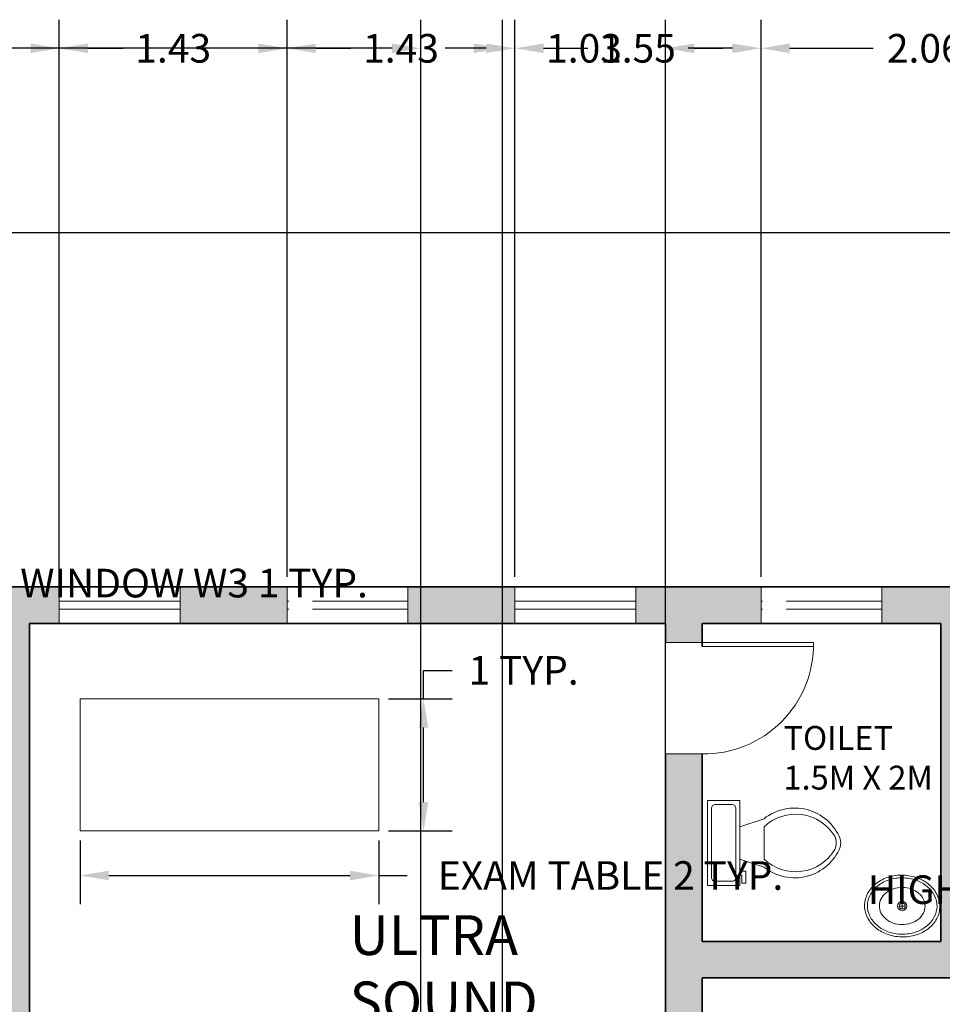
# Model space of a CAD drawing. Units: metres. Extents: x 4298.5 to 4325.2, y 2075 to 2095.8.
# Tile 34 of 35: x 4314.3 to 4320.1, y 2089.6 to 2095.8. Entities that reach past the tile are written whole.
import ezdxf

# ---------------------------------------------------------------- set-up
doc = ezdxf.new("R2010")
doc.units = ezdxf.units.M
doc.linetypes.add('ACAD_ISO02W100', pattern=[15, 12, -3])
for name, color, linetype, lineweight in [('A-ANNO-DIMS', 2, 'Continuous', 18), ('A-AREA-IDEN', 7, 'Continuous', 18), ('A-DOOR', 3, 'Continuous', 18), ('A-EQPM', 9, 'Continuous', 18), ('A-FLOR-FIXT', 15, 'Continuous', 18), ('A-GLAZ', 4, 'Continuous', 18), ('A-GLAZ-OVHD', 4, 'ACAD_ISO02W100', 13), ('A-WALL', 7, 'Continuous', 35), ('A-WALL-PATT', 252, 'Continuous', 13)]:
    doc.layers.add(name, color=color, linetype=linetype, lineweight=lineweight)
doc.styles.get("Standard").update_dxf_attribs({"font": 'arial.ttf'})
doc.dimstyles.get("Standard").update_dxf_attribs({"dimtxt": 0.18, "dimasz": 0.18, "dimexe": 0.18, "dimexo": 0.0625, "dimgap": 0.09, "dimtad": 0, "dimtih": 1, "dimtoh": 1, "dimdec": 4, "dimzin": 0, "dimdsep": 46, "dimtxsty": 'Standard', "dimcen": 0.09, "dimadec": 0, "dimazin": 0, "dimtfac": 1, "dimtdec": 4, "dimtofl": 0, "dimtmove": 0, "dimatfit": 3, "dimfxl": 1, "dimtolj": 1, "dimtzin": 0, "dimarcsym": 0})

# ---------------------------------------------------------------- blocks, each defined once
blk = doc.blocks.new('Toilet - top')
for p, q in [((9.5, -6), (9.5, -2)), ((-10, -8.5), (-8, -8.5)), ((-10, -9.5), (-10, -8.5)), ((-7, -9.5), (-10, -9.5)), ((-8, -8.5), (-8, -8)), ((-7, -8), (-7, -9.5)), ((-4, -8), (-6, -14)), ((4, -8), (6, -14)), ((4, -14), (-4, -14))]:
    blk.add_line(p, q)
blk.add_lwpolyline([(10.5, -8), (10.5, 0), (-10.5, 0), (-10.5, -8)], close=True)
for points in [[(-9.5, -2), (-9.5, -6)], [(8.5, -1), (-8.5, -1)], [(-8.5, -7), (8.5, -7)]]:
    blk.add_lwpolyline(points)
for centre, radius, start, end in [((-8.62, -1.88), 0.884, 81.8699, 188.1301), ((8.62, -1.88), 0.884, 351.8699, 98.1301), ((-8.62, -6.12), 0.884, 171.8699, 278.1301), ((8.62, -6.12), 0.884, 261.8699, 8.1301), ((3.52, -21.58), 12.17, 141.4691, 247.9714), ((4.2, -21.82), 11.33, 136.3677, 238.9468), ((-3.52, -21.58), 12.17, 292.0284, 38.5307), ((-4.2, -21.82), 11.33, 301.053, 43.6321), ((0, -27.88), 4, 245.7318, 294.2682), ((0, -29), 4, 254.8605, 285.1395)]:
    blk.add_arc(centre, radius, start, end)
blk = doc.blocks.new('Sink - Oval top')
for p, q in [((-1, 0), (1, 0)), ((0, 1), (0, -1))]:
    blk.add_line(p, q)
for points in [[(-12.23, 0.39, 0.117634), (-11.46, -3.36, 0.104469), (-8.88, -6.8, 0.090016), (-5.08, -9.07, 0.08192), (-0.32, -10.02, 0.08192), (4.49, -9.38, 0.090016), (8.42, -7.36, 0.104469), (11.22, -4.09, 0.117634), (12.23, -0.39, 0.117634), (11.46, 3.36, 0.104469), (8.88, 6.8, 0.090016), (5.08, 9.07, 0.08192), (0.32, 10.02, 0.08192), (-4.49, 9.38, 0.090016), (-8.42, 7.36, 0.104469), (-11.22, 4.09, 0.117634)], [(-11.29, 0.16, 0.118622), (-10.52, -3.25, 0.104678), (-8.07, -6.36, 0.089562), (-4.54, -8.37, 0.081185), (-0.13, -9.15, 0.081185), (4.3, -8.49, 0.089562), (7.89, -6.58, 0.104678), (10.42, -3.55, 0.118622), (11.29, -0.16, 0.118622), (10.52, 3.25, 0.104678), (8.07, 6.36, 0.089562), (4.54, 8.37, 0.081185), (0.13, 9.15, 0.081185), (-4.3, 8.49, 0.089562), (-7.89, 6.58, 0.104678), (-10.42, 3.55, 0.118622)], [(-7.42, 0.08, 0.118283), (-6.91, -2.17, 0.104607), (-5.29, -4.21, 0.089718), (-2.97, -5.53, 0.081436), (-0.07, -6.04, 0.081436), (2.84, -5.59, 0.089718), (5.2, -4.33, 0.104607), (6.86, -2.32, 0.118283), (7.42, -0.08, 0.118283), (6.91, 2.17, 0.104607), (5.29, 4.21, 0.089718), (2.97, 5.53, 0.081436), (0.07, 6.04, 0.081436), (-2.84, 5.59, 0.089718), (-5.2, 4.33, 0.104607), (-6.86, 2.32, 0.118283)]]:
    blk.add_lwpolyline(points, format="xyb", close=True)
for radius in [1.5, 1]:
    blk.add_circle((0, 0), radius)
blk = doc.blocks.new('WIN-760-GLASS-HIGH')
at = {"ltscale": 0.05}
for p, q in [((0, 0.76), (0, 0)), ((0.05, 0.76), (0.05, 0))]:
    blk.add_line(p, q, dxfattribs=at)
blk = doc.blocks.new('WIN-760-GLASS')
for p, q in [((0, 0.76), (0, 0)), ((0.05, 0.76), (0.05, 0))]:
    blk.add_line(p, q)
blk = doc.blocks.new('DOOR-700-LEAF')
for p, q in [((0.675, 0), (0.675, 0.7)), ((0.7, 0), (0.7, 0.7))]:
    blk.add_line(p, q)
blk.add_arc((0.6875, 0.0125), 0.6876, 88.95837, 181.04163)
blk = doc.blocks.new('EXAM-TABLE-1880')
blk.add_lwpolyline([(0, 0.8289), (1.8779, 0.8289), (1.8779, 0), (0, 0)], close=True)
blk = doc.blocks.new('*D25')
at = {"layer": 'A-ANNO-DIMS', "color": 0, "lineweight": -2, "transparency": 16777216}
for p, q in [((4322.7831, 2091.2831), (4323.0146, 2091.2831)), ((4322.8346, 2091.1031), (4322.8346, 2090.7031)), ((4322.7831, 2090.5231), (4323.0146, 2090.5231)), ((4322.8346, 2090.5231), (4322.8346, 2090.3431)), ((4322.8346, 2090.3431), (4322.6546, 2090.3431))]:
    blk.add_line(p, q, dxfattribs=at)
at = {"layer": 'A-ANNO-DIMS', "color": 0, "transparency": 16777216}
for points in [[(4322.8046, 2091.1031), (4322.8646, 2091.1031), (4322.8346, 2091.2831)], [(4322.8046, 2090.7031), (4322.8646, 2090.7031), (4322.8346, 2090.5231)]]:
    blk.add_solid(points, dxfattribs=at)
at = {"layer": 'Defpoints', "color": 0, "transparency": 16777216}
for p in [(4322.7206, 2091.2831), (4322.7206, 2090.5231), (4322.8346, 2090.5231)]:
    blk.add_point(p, dxfattribs=at)
at = {"layer": 'A-ANNO-DIMS', "color": 0, "transparency": 16777216, "insert": (4321.0419, 2090.3431), "char_height": 0.18, "attachment_point": 5}
blk.add_mtext('\\A1;HIGH WINDOW W2 1 TYP.', dxfattribs=at)
blk = doc.blocks.new('*D27')
at = {"layer": 'A-ANNO-DIMS', "color": 0, "lineweight": -2, "transparency": 16777216}
for p, q in [((4313.1733, 2092.2206), (4313.1733, 2092.4521)), ((4313.9333, 2092.2206), (4313.9333, 2092.4521)), ((4313.3533, 2092.2721), (4313.7533, 2092.2721)), ((4313.9333, 2092.2721), (4314.1133, 2092.2721))]:
    blk.add_line(p, q, dxfattribs=at)
at = {"layer": 'A-ANNO-DIMS', "color": 0, "transparency": 16777216}
for points in [[(4313.3533, 2092.3021), (4313.3533, 2092.2421), (4313.1733, 2092.2721)], [(4313.7533, 2092.3021), (4313.7533, 2092.2421), (4313.9333, 2092.2721)]]:
    blk.add_solid(points, dxfattribs=at)
at = {"layer": 'Defpoints', "color": 0, "transparency": 16777216}
for p in [(4313.9333, 2092.2721), (4313.1733, 2092.1581), (4313.9333, 2092.1581)]:
    blk.add_point(p, dxfattribs=at)
at = {"layer": 'A-ANNO-DIMS', "color": 0, "transparency": 16777216, "insert": (4315.3853, 2092.2721), "char_height": 0.18, "attachment_point": 5}
blk.add_mtext('\\A1;WINDOW W3 1 TYP.', dxfattribs=at)
blk = doc.blocks.new('*D41')
at = {"layer": 'A-ANNO-DIMS', "color": 0, "lineweight": -2, "transparency": 16777216}
for p, q in [((4314.6686, 2090.6517), (4314.6686, 2090.2525)), ((4316.5464, 2090.6517), (4316.5464, 2090.2525)), ((4314.8486, 2090.4325), (4316.3664, 2090.4325)), ((4316.5464, 2090.4325), (4316.7264, 2090.4325))]:
    blk.add_line(p, q, dxfattribs=at)
at = {"layer": 'A-ANNO-DIMS', "color": 0, "transparency": 16777216}
for points in [[(4314.8486, 2090.4625), (4314.8486, 2090.4025), (4314.6686, 2090.4325)], [(4316.3664, 2090.4625), (4316.3664, 2090.4025), (4316.5464, 2090.4325)]]:
    blk.add_solid(points, dxfattribs=at)
at = {"layer": 'Defpoints', "color": 0, "transparency": 16777216}
for p in [(4314.6686, 2090.7142), (4316.5464, 2090.7142), (4316.5464, 2090.4325)]:
    blk.add_point(p, dxfattribs=at)
at = {"layer": 'A-ANNO-DIMS', "color": 0, "transparency": 16777216, "insert": (4318.0043, 2090.4325), "char_height": 0.18, "attachment_point": 5}
blk.add_mtext('\\A1;EXAM TABLE 2 TYP.', dxfattribs=at)
blk = doc.blocks.new('*D42')
at = {"layer": 'A-ANNO-DIMS', "color": 0, "lineweight": -2, "transparency": 16777216}
for p, q in [((4316.8281, 2091.543), (4316.8281, 2091.723)), ((4316.8281, 2091.723), (4317.0081, 2091.723)), ((4316.6089, 2091.543), (4317.0081, 2091.543)), ((4316.8281, 2090.8942), (4316.8281, 2091.363)), ((4316.6089, 2090.7142), (4317.0081, 2090.7142))]:
    blk.add_line(p, q, dxfattribs=at)
at = {"layer": 'A-ANNO-DIMS', "color": 0, "transparency": 16777216}
for points in [[(4316.7981, 2091.363), (4316.8581, 2091.363), (4316.8281, 2091.543)], [(4316.7981, 2090.8942), (4316.8581, 2090.8942), (4316.8281, 2090.7142)]]:
    blk.add_solid(points, dxfattribs=at)
at = {"layer": 'Defpoints', "color": 0, "transparency": 16777216}
for p in [(4316.5464, 2091.543), (4316.8281, 2091.543), (4316.5464, 2090.7142)]:
    blk.add_point(p, dxfattribs=at)
at = {"layer": 'A-ANNO-DIMS', "color": 0, "transparency": 16777216, "insert": (4317.4578, 2091.723), "char_height": 0.18, "attachment_point": 5}
blk.add_mtext('\\A1;1 TYP.', dxfattribs=at)
blk = doc.blocks.new('*D48')
at = {"layer": 'A-ANNO-DIMS', "color": 0, "lineweight": -2, "transparency": 16777216}
for p, q in [((4310.1831, 2094.4781), (4324.7671, 2094.4781)), ((4324.5871, 2094.2981), (4324.5871, 2085.585)), ((4324.5871, 2076.5081), (4324.5871, 2085.2212)), ((4316.8731, 2076.3281), (4324.7671, 2076.3281))]:
    blk.add_line(p, q, dxfattribs=at)
at = {"layer": 'A-ANNO-DIMS', "color": 0, "transparency": 16777216}
for points in [[(4324.5571, 2094.2981), (4324.6171, 2094.2981), (4324.5871, 2094.4781)], [(4324.5571, 2076.5081), (4324.6171, 2076.5081), (4324.5871, 2076.3281)]]:
    blk.add_solid(points, dxfattribs=at)
at = {"layer": 'Defpoints', "color": 0, "transparency": 16777216}
for p in [(4310.1206, 2094.4781), (4316.8106, 2076.3281), (4324.5871, 2076.3281)]:
    blk.add_point(p, dxfattribs=at)
at = {"layer": 'A-ANNO-DIMS', "color": 0, "transparency": 16777216, "insert": (4324.5871, 2085.4031), "char_height": 0.18, "attachment_point": 5}
blk.add_mtext('\\A1;18.15', dxfattribs=at)
blk = doc.blocks.new('*D53')
at = {"layer": 'A-ANNO-DIMS', "color": 0, "lineweight": -2, "transparency": 16777216}
for p, q in [((4309.1606, 2076.3906), (4309.1606, 2095.8166)), ((4316.8106, 2076.3906), (4316.8106, 2095.8166)), ((4309.3406, 2095.6366), (4312.6619, 2095.6366)), ((4316.6306, 2095.6366), (4313.3093, 2095.6366))]:
    blk.add_line(p, q, dxfattribs=at)
at = {"layer": 'A-ANNO-DIMS', "color": 0, "transparency": 16777216}
for points in [[(4309.3406, 2095.6666), (4309.3406, 2095.6066), (4309.1606, 2095.6366)], [(4316.6306, 2095.6666), (4316.6306, 2095.6066), (4316.8106, 2095.6366)]]:
    blk.add_solid(points, dxfattribs=at)
at = {"layer": 'Defpoints', "color": 0, "transparency": 16777216}
for p in [(4316.8106, 2095.6366), (4309.1606, 2076.3281), (4316.8106, 2076.3281)]:
    blk.add_point(p, dxfattribs=at)
at = {"layer": 'A-ANNO-DIMS', "color": 0, "transparency": 16777216, "insert": (4312.9856, 2095.6366), "char_height": 0.18, "attachment_point": 5}
blk.add_mtext('\\A1;7.65', dxfattribs=at)
blk = doc.blocks.new('*D61')
at = {"layer": 'A-ANNO-DIMS', "color": 0, "lineweight": -2, "transparency": 16777216}
for p, q in [((4317.324045, 2083.575187), (4317.324045, 2095.816556)), ((4318.350577, 2084.620556), (4318.350577, 2095.816556)), ((4317.144045, 2095.636556), (4316.964045, 2095.636556)), ((4318.530577, 2095.636556), (4318.710577, 2095.636556))]:
    blk.add_line(p, q, dxfattribs=at)
at = {"layer": 'A-ANNO-DIMS', "color": 0, "transparency": 16777216}
for points in [[(4317.144045, 2095.666556), (4317.144045, 2095.606556), (4317.324045, 2095.636556)], [(4318.530577, 2095.666556), (4318.530577, 2095.606556), (4318.350577, 2095.636556)]]:
    blk.add_solid(points, dxfattribs=at)
at = {"layer": 'Defpoints', "color": 0, "transparency": 16777216}
for p in [(4318.350577, 2095.636556), (4318.350577, 2084.558056), (4317.324045, 2083.512687)]:
    blk.add_point(p, dxfattribs=at)
at = {"layer": 'A-ANNO-DIMS', "color": 0, "transparency": 16777216, "insert": (4317.837311, 2095.636556), "char_height": 0.18, "attachment_point": 5}
blk.add_mtext('\\A1;1.03', dxfattribs=at)
blk = doc.blocks.new('*D68')
at = {"layer": 'A-ANNO-DIMS', "color": 0, "lineweight": -2, "transparency": 16777216}
for p, q in [((4313.1733, 2092.3106), (4313.1733, 2095.8166)), ((4314.5378, 2092.3106), (4314.5378, 2095.8166)), ((4313.3533, 2095.6366), (4313.5403, 2095.6366)), ((4314.3578, 2095.6366), (4314.1708, 2095.6366))]:
    blk.add_line(p, q, dxfattribs=at)
at = {"layer": 'A-ANNO-DIMS', "color": 0, "transparency": 16777216}
for points in [[(4313.3533, 2095.6666), (4313.3533, 2095.6066), (4313.1733, 2095.6366)], [(4314.3578, 2095.6666), (4314.3578, 2095.6066), (4314.5378, 2095.6366)]]:
    blk.add_solid(points, dxfattribs=at)
at = {"layer": 'Defpoints', "color": 0, "transparency": 16777216}
for p in [(4314.5378, 2095.6366), (4313.1733, 2092.2481), (4314.5378, 2092.2481)]:
    blk.add_point(p, dxfattribs=at)
at = {"layer": 'A-ANNO-DIMS', "color": 0, "transparency": 16777216, "insert": (4313.8556, 2095.6366), "char_height": 0.18, "attachment_point": 5}
blk.add_mtext('\\A1;1.36', dxfattribs=at)
blk = doc.blocks.new('*D69')
at = {"layer": 'A-ANNO-DIMS', "color": 0, "lineweight": -2, "transparency": 16777216}
for p, q in [((4314.5378, 2092.3106), (4314.5378, 2095.8166)), ((4315.9706, 2092.3106), (4315.9706, 2095.8166)), ((4314.7178, 2095.6366), (4314.9389, 2095.6366)), ((4315.7906, 2095.6366), (4315.5695, 2095.6366))]:
    blk.add_line(p, q, dxfattribs=at)
at = {"layer": 'A-ANNO-DIMS', "color": 0, "transparency": 16777216}
for points in [[(4314.7178, 2095.6666), (4314.7178, 2095.6066), (4314.5378, 2095.6366)], [(4315.7906, 2095.6666), (4315.7906, 2095.6066), (4315.9706, 2095.6366)]]:
    blk.add_solid(points, dxfattribs=at)
at = {"layer": 'Defpoints', "color": 0, "transparency": 16777216}
for p in [(4315.9706, 2095.6366), (4314.5378, 2092.2481), (4315.9706, 2092.2481)]:
    blk.add_point(p, dxfattribs=at)
at = {"layer": 'A-ANNO-DIMS', "color": 0, "transparency": 16777216, "insert": (4315.2542, 2095.6366), "char_height": 0.18, "attachment_point": 5}
blk.add_mtext('\\A1;1.43', dxfattribs=at)
blk = doc.blocks.new('*D70')
at = {"layer": 'A-ANNO-DIMS', "color": 0, "lineweight": -2, "transparency": 16777216}
for p, q in [((4315.9706, 2092.3106), (4315.9706, 2095.8166)), ((4317.4033, 2092.3106), (4317.4033, 2095.8166)), ((4316.1506, 2095.6366), (4316.3716, 2095.6366)), ((4317.2233, 2095.6366), (4317.0022, 2095.6366))]:
    blk.add_line(p, q, dxfattribs=at)
at = {"layer": 'A-ANNO-DIMS', "color": 0, "transparency": 16777216}
for points in [[(4316.1506, 2095.6666), (4316.1506, 2095.6066), (4315.9706, 2095.6366)], [(4317.2233, 2095.6666), (4317.2233, 2095.6066), (4317.4033, 2095.6366)]]:
    blk.add_solid(points, dxfattribs=at)
at = {"layer": 'Defpoints', "color": 0, "transparency": 16777216}
for p in [(4317.4033, 2095.6366), (4315.9706, 2092.2481), (4317.4033, 2092.2481)]:
    blk.add_point(p, dxfattribs=at)
at = {"layer": 'A-ANNO-DIMS', "color": 0, "transparency": 16777216, "insert": (4316.6869, 2095.6366), "char_height": 0.18, "attachment_point": 5}
blk.add_mtext('\\A1;1.43', dxfattribs=at)
blk = doc.blocks.new('*D71')
at = {"layer": 'A-ANNO-DIMS', "color": 0, "lineweight": -2, "transparency": 16777216}
for p, q in [((4317.4033, 2092.3106), (4317.4033, 2095.8166)), ((4318.9506, 2092.3106), (4318.9506, 2095.8166)), ((4317.5833, 2095.6366), (4317.861, 2095.6366)), ((4318.7706, 2095.6366), (4318.4929, 2095.6366))]:
    blk.add_line(p, q, dxfattribs=at)
at = {"layer": 'A-ANNO-DIMS', "color": 0, "transparency": 16777216}
for points in [[(4317.5833, 2095.6666), (4317.5833, 2095.6066), (4317.4033, 2095.6366)], [(4318.7706, 2095.6666), (4318.7706, 2095.6066), (4318.9506, 2095.6366)]]:
    blk.add_solid(points, dxfattribs=at)
at = {"layer": 'Defpoints', "color": 0, "transparency": 16777216}
for p in [(4318.9506, 2095.6366), (4317.4033, 2092.2481), (4318.9506, 2092.2481)]:
    blk.add_point(p, dxfattribs=at)
at = {"layer": 'A-ANNO-DIMS', "color": 0, "transparency": 16777216, "insert": (4318.1769, 2095.6366), "char_height": 0.18, "attachment_point": 5}
blk.add_mtext('\\A1;1.55', dxfattribs=at)
blk = doc.blocks.new('*D72')
at = {"layer": 'A-ANNO-DIMS', "color": 0, "lineweight": -2, "transparency": 16777216}
for p, q in [((4318.9506, 2092.3106), (4318.9506, 2095.8166)), ((4321.0106, 2092.3106), (4321.0106, 2095.8166)), ((4319.1306, 2095.6366), (4319.6553, 2095.6366)), ((4320.8306, 2095.6366), (4320.3058, 2095.6366))]:
    blk.add_line(p, q, dxfattribs=at)
at = {"layer": 'A-ANNO-DIMS', "color": 0, "transparency": 16777216}
for points in [[(4319.1306, 2095.6666), (4319.1306, 2095.6066), (4318.9506, 2095.6366)], [(4320.8306, 2095.6666), (4320.8306, 2095.6066), (4321.0106, 2095.6366)]]:
    blk.add_solid(points, dxfattribs=at)
at = {"layer": 'Defpoints', "color": 0, "transparency": 16777216}
for p in [(4321.0106, 2095.6366), (4318.9506, 2092.2481), (4321.0106, 2092.2481)]:
    blk.add_point(p, dxfattribs=at)
at = {"layer": 'A-ANNO-DIMS', "color": 0, "transparency": 16777216, "insert": (4319.9806, 2095.6366), "char_height": 0.18, "attachment_point": 5}
blk.add_mtext('\\A1;2.06', dxfattribs=at)

msp = doc.modelspace()

# ---------------------------------------------------------------- hatches: boundary and pattern name
at = {"layer": 'A-WALL-PATT'}
h = msp.add_hatch(color=256, dxfattribs=at)
h.dxf.hatch_style = 1
h.paths.add_polyline_path([(4308.7606, 2094.4781), (4308.1606, 2094.4781), (4307.4606, 2094.4781), (4307.4606, 2094.2481), (4308.2706, 2094.2481), (4308.2706, 2094.1281), (4308.3906, 2094.1281), (4308.3906, 2094.2481), (4308.7606, 2094.2481)])
h.paths.add_polyline_path([(4310.1206, 2094.4781), (4309.5206, 2094.4781), (4309.5206, 2094.2481), (4309.8906, 2094.2481), (4309.8906, 2092.2481), (4308.3906, 2092.2481), (4308.3906, 2093.4281), (4308.2706, 2093.4281), (4308.2706, 2092.0181), (4309.8906, 2092.0181), (4309.8906, 2087.0181), (4309.7706, 2087.0181), (4309.7706, 2086.7881), (4309.8906, 2086.7881), (4311.9406, 2086.7881), (4311.9406, 2087.0181), (4310.1206, 2087.0181), (4310.1206, 2089.0181), (4310.2406, 2089.0181), (4310.2406, 2089.1381), (4310.1206, 2089.1381), (4310.1206, 2092.0181), (4310.3078, 2092.0181), (4310.3078, 2092.2481), (4310.1206, 2092.2481)])
h.paths.add_polyline_path([(4311.7406, 2092.2481), (4311.0678, 2092.2481), (4311.0678, 2092.0181), (4311.7406, 2092.0181)], flags=17)
h.paths.add_polyline_path([(4313.1733, 2092.2481), (4312.5006, 2092.2481), (4312.5006, 2092.0181), (4313.1733, 2092.0181)])
h.paths.add_polyline_path([(4314.5378, 2092.2481), (4314.1206, 2092.2481), (4313.9333, 2092.2481), (4313.9333, 2092.0181), (4314.1206, 2092.0181), (4314.1206, 2087.0181), (4314.0006, 2087.0181), (4314.0006, 2086.7881), (4314.1206, 2086.7881), (4315.5718, 2086.7881), (4315.5718, 2087.0181), (4314.3506, 2087.0181), (4314.3506, 2092.0181), (4314.5378, 2092.0181)])
h.paths.add_polyline_path([(4315.9706, 2092.2481), (4315.2978, 2092.2481), (4315.2978, 2092.0181), (4315.9706, 2092.0181)])
h.paths.add_polyline_path([(4317.4033, 2092.2481), (4316.7306, 2092.2481), (4316.7306, 2092.0181), (4317.4033, 2092.0181)])
h.paths.add_polyline_path([(4318.9506, 2092.2481), (4318.3506, 2092.2481), (4318.1633, 2092.2481), (4318.1633, 2092.0181), (4318.3506, 2092.0181), (4318.3506, 2091.8981), (4318.5806, 2091.8981), (4318.5806, 2092.0181), (4318.9506, 2092.0181)])
h.paths.add_polyline_path([(4321.0106, 2092.2481), (4319.7106, 2092.2481), (4319.7106, 2092.0181), (4320.0806, 2092.0181), (4320.0806, 2090.0181), (4318.5806, 2090.0181), (4318.5806, 2091.1981), (4318.3506, 2091.1981), (4318.3506, 2090.0181), (4318.3506, 2087.0181), (4318.2306, 2087.0181), (4318.2306, 2086.7881), (4318.3506, 2086.7881), (4318.3506, 2086.3081), (4318.5806, 2086.3081), (4318.5806, 2089.7881), (4321.7806, 2089.7881), (4321.7806, 2090.0181), (4320.2006, 2090.0181), (4320.2006, 2092.0181), (4321.0106, 2092.0181)])
h.paths.add_polyline_path([(4322.8106, 2092.2481), (4321.7706, 2092.2481), (4321.7706, 2092.0181), (4322.5806, 2092.0181), (4322.5806, 2091.2831), (4322.8106, 2091.2831)])
h.paths.add_polyline_path([(4322.8106, 2090.5231), (4322.5806, 2090.5231), (4322.5806, 2089.7881), (4322.5806, 2089.5254), (4322.8106, 2089.5254), (4322.8106, 2090.0181)])
h.paths.add_polyline_path([(4322.8106, 2088.7654), (4322.5806, 2088.7654), (4322.5806, 2087.6681), (4322.8106, 2087.6681)])
h.paths.add_polyline_path([(4322.8106, 2086.9081), (4322.5806, 2086.9081), (4322.5806, 2085.8107), (4322.8106, 2085.8107)])
h.paths.add_polyline_path([(4322.8106, 2085.0507), (4322.5806, 2085.0507), (4322.5806, 2084.7881), (4318.5806, 2084.7881), (4318.5806, 2085.0581), (4318.5806, 2085.4081), (4318.3506, 2085.4081), (4318.3506, 2084.5581), (4318.3506, 2080.8581), (4318.4706, 2080.8581), (4318.4706, 2082.3281), (4319.2606, 2082.3281), (4319.2606, 2082.5581), (4318.5806, 2082.5581), (4318.5806, 2084.5581), (4320.0806, 2084.5581), (4320.0806, 2083.9381), (4320.3106, 2083.9381), (4320.3106, 2084.5581), (4322.8106, 2084.5581)])
h.paths.add_polyline_path([(4320.3106, 2083.1781), (4320.0806, 2083.1781), (4320.0806, 2082.5581), (4319.9606, 2082.5581), (4319.9606, 2082.3281), (4320.0806, 2082.3281), (4320.0806, 2081.5731), (4320.3106, 2081.5731)], flags=17)
h.paths.add_polyline_path([(4320.3106, 2080.8131), (4320.0806, 2080.8131), (4320.0806, 2080.0581), (4318.4286, 2080.0581), (4318.4286, 2079.8281), (4320.3106, 2079.8281)])
h.paths.add_polyline_path([(4317.3506, 2085.2881), (4316.5718, 2085.2881), (4316.5718, 2085.0581), (4317.3506, 2085.0581)])
h.paths.add_polyline_path([(4315.5718, 2085.2881), (4314.8434, 2085.2881), (4314.8434, 2085.0581), (4315.5718, 2085.0581)])
h.paths.add_polyline_path([(4313.8434, 2085.2881), (4312.9406, 2085.2881), (4312.9406, 2085.0581), (4313.8434, 2085.0581)])
h.paths.add_polyline_path([(4311.9406, 2085.2881), (4311.4406, 2085.2881), (4311.4406, 2085.0581), (4311.9406, 2085.0581)])
h.paths.add_polyline_path([(4317.3306, 2087.0181), (4316.5718, 2087.0181), (4316.5718, 2086.7881), (4317.3306, 2086.7881)])
h.paths.add_polyline_path([(4313.1006, 2089.1381), (4311.1406, 2089.1381), (4311.1406, 2089.0181), (4312.9806, 2089.0181), (4312.9806, 2087.0181), (4312.9406, 2087.0181), (4312.9406, 2086.7881), (4313.1006, 2086.7881), (4313.1006, 2087.0181)])
h.paths.add_polyline_path([(4307.5515, 2087.0181), (4305.8906, 2087.0181), (4305.8906, 2092.2481), (4305.8906, 2094.2481), (4306.7006, 2094.2481), (4306.7006, 2094.4781), (4305.6606, 2094.4781), (4305.6606, 2092.2481), (4305.2906, 2092.2481), (4305.2906, 2092.0181), (4305.6606, 2092.0181), (4305.6606, 2090.0181), (4304.1606, 2090.0181), (4304.1606, 2091.1981), (4304.0406, 2091.1981), (4304.0406, 2089.9081), (4301.5606, 2089.9081), (4301.5606, 2089.7881), (4304.0406, 2089.7881), (4305.6606, 2089.7881), (4305.6606, 2086.6381), (4305.8906, 2086.6381), (4305.8906, 2086.7881), (4307.5515, 2086.7881)])
h.paths.add_polyline_path([(4307.5515, 2085.2881), (4305.8906, 2085.2881), (4305.8906, 2085.4381), (4305.6606, 2085.4381), (4305.6606, 2084.7881), (4305.2906, 2084.7881), (4305.2906, 2084.5581), (4305.6606, 2084.5581), (4305.6606, 2084.02), (4305.8906, 2084.02), (4305.8906, 2084.5581), (4305.8906, 2085.0581), (4307.5515, 2085.0581)])
h.paths.add_polyline_path([(4310.2406, 2085.2881), (4308.5515, 2085.2881), (4308.5515, 2085.0581), (4310.2406, 2085.0581)])
h.paths.add_polyline_path([(4317.4286, 2080.0581), (4316.5718, 2080.0581), (4316.5718, 2079.8281), (4317.4286, 2079.8281)])
h.paths.add_polyline_path([(4315.5718, 2080.0581), (4314.8434, 2080.0581), (4314.8434, 2079.8281), (4315.5718, 2079.8281)])
h.paths.add_polyline_path([(4313.8434, 2080.0581), (4312.9406, 2080.0581), (4312.9406, 2079.8281), (4313.8434, 2079.8281)])
h.paths.add_polyline_path([(4311.9406, 2080.0581), (4311.4406, 2080.0581), (4311.4406, 2079.8281), (4311.9406, 2079.8281)])
h.paths.add_polyline_path([(4310.2406, 2080.0581), (4310.1206, 2080.0581), (4310.1206, 2084.0381), (4309.8906, 2084.0381), (4309.8906, 2080.0581), (4309.1606, 2080.0581), (4309.1606, 2079.8281), (4310.2406, 2079.8281)])
h.paths.add_polyline_path([(4308.1606, 2080.0581), (4307.5106, 2080.0581), (4307.5106, 2080.1781), (4307.3906, 2080.1781), (4307.3906, 2080.0581), (4305.8906, 2080.0581), (4305.8906, 2080.567), (4305.6606, 2080.567), (4305.6606, 2079.8281), (4308.1606, 2079.8281)])
h.paths.add_polyline_path([(4307.5106, 2081.9381), (4309.0906, 2081.9381), (4309.0906, 2082.0581), (4305.8906, 2082.0581), (4305.8906, 2083.26), (4305.6606, 2083.26), (4305.6606, 2081.327), (4305.8906, 2081.327), (4305.8906, 2081.9381), (4307.3906, 2081.9381), (4307.3906, 2080.8781), (4307.5106, 2080.8781)])
h.paths.add_polyline_path([(4304.5306, 2084.7881), (4302.7306, 2084.7881), (4302.7306, 2084.5581), (4304.5306, 2084.5581)])
h.paths.add_polyline_path([(4301.9706, 2084.7881), (4300.6606, 2084.7881), (4300.6606, 2085.0249), (4300.4306, 2085.0249), (4300.4306, 2084.5581), (4301.9706, 2084.5581)])
h.paths.add_polyline_path([(4300.6606, 2086.8843), (4300.4306, 2086.8843), (4300.4306, 2085.7849), (4300.6606, 2085.7849)])
h.paths.add_polyline_path([(4300.6606, 2089.1618), (4300.4306, 2089.1618), (4300.4306, 2087.6443), (4300.6606, 2087.6443)])
h.paths.add_polyline_path([(4300.6606, 2091.0212), (4300.4306, 2091.0212), (4300.4306, 2089.9218), (4300.6606, 2089.9218)])
h.paths.add_polyline_path([(4300.6606, 2092.0181), (4301.9706, 2092.0181), (4301.9706, 2092.2481), (4300.4306, 2092.2481), (4300.4306, 2091.7812), (4300.6606, 2091.7812)])
h.paths.add_polyline_path([(4304.5306, 2092.2481), (4302.7306, 2092.2481), (4302.7306, 2092.0181), (4304.0406, 2092.0181), (4304.0406, 2091.8981), (4304.1606, 2091.8981), (4304.1606, 2092.0181), (4304.5306, 2092.0181)], flags=17)

# ---------------------------------------------------------------- linework, layer by layer
at = {"layer": 'A-DOOR'}
for p, q in [((4318.5806, 2091.8981), (4318.3506, 2091.8981)), ((4318.5806, 2091.1981), (4318.3506, 2091.1981))]:
    msp.add_line(p, q, dxfattribs=at)
at = {"layer": 'A-GLAZ'}
for p, q in [((4314.5378, 2092.0181), (4314.5378, 2092.2481)), ((4315.2978, 2092.0181), (4315.2978, 2092.2481)), ((4315.9706, 2092.0181), (4315.9706, 2092.2481)), ((4316.7306, 2092.0181), (4316.7306, 2092.2481)), ((4317.4033, 2092.0181), (4317.4033, 2092.2481)), ((4318.1633, 2092.0181), (4318.1633, 2092.2481)), ((4318.9506, 2092.0181), (4318.9506, 2092.2481)), ((4319.7106, 2092.0181), (4319.7106, 2092.2481))]:
    msp.add_line(p, q, dxfattribs=at)
at = {"layer": 'A-WALL'}
for p, q in [((4318.3506, 2092.2481), (4314.1206, 2092.2481)), ((4318.3506, 2092.2481), (4322.8106, 2092.2481)), ((4318.3506, 2092.0181), (4314.3506, 2092.0181)), ((4314.3506, 2092.0181), (4314.3506, 2087.0181)), ((4318.3506, 2091.8981), (4318.3506, 2092.0181)), ((4318.5806, 2092.0181), (4320.0806, 2092.0181)), ((4318.5806, 2091.8731), (4318.5806, 2092.0181)), ((4320.0806, 2090.0181), (4320.0806, 2092.0181)), ((4318.3506, 2090.0181), (4318.3506, 2091.1981)), ((4318.5806, 2090.0181), (4318.5806, 2091.1981)), ((4318.3506, 2087.0181), (4318.3506, 2090.0181)), ((4318.5806, 2090.0181), (4320.0806, 2090.0181)), ((4318.5806, 2089.7881), (4321.7806, 2089.7881)), ((4318.5806, 2086.3081), (4318.5806, 2089.7881))]:
    msp.add_line(p, q, dxfattribs=at)

# ---------------------------------------------------------------- block references
at = {"layer": 'A-DOOR', "extrusion": (0, 0, -1), "zscale": -1, "rotation": 89.99999999999999}
msp.add_blockref('DOOR-700-LEAF', (-4318.5806, 2091.198), dxfattribs=at)
at = {"layer": 'A-EQPM'}
msp.add_blockref('EXAM-TABLE-1880', (4314.6686, 2090.7142), dxfattribs=at)
at = {"layer": 'A-FLOR-FIXT', "xscale": 0.0254, "yscale": 0.0254, "zscale": 0.0254, "rotation": 90.00015040587188}
msp.add_blockref('Toilet - top', (4318.6139, 2090.6373), dxfattribs=at)
at = {"layer": 'A-FLOR-FIXT', "xscale": 0.0193818050953029, "yscale": 0.0193818050953029, "zscale": 0.0193818050953029}
msp.add_blockref('Sink - Oval top', (4319.8385, 2090.2405), dxfattribs=at)
at = {"layer": 'A-GLAZ'}
for p, rotation in [((4314.5378, 2092.1581), 269.9999999999362), ((4317.4033, 2092.1581), 269.9999999999272)]:
    msp.add_blockref('WIN-760-GLASS', p, dxfattribs=dict(at, rotation=rotation))
at = {"layer": 'A-GLAZ-OVHD'}
for p, rotation in [((4315.9706, 2092.1581), 269.9999999999317), ((4318.9506, 2092.1581), 269.9999999999227)]:
    msp.add_blockref('WIN-760-GLASS-HIGH', p, dxfattribs=dict(at, rotation=rotation))

# ---------------------------------------------------------------- texts
at = {"layer": 'A-AREA-IDEN', "attachment_point": 1}
for s, insert, char_height in [('TOILET\\P1.5M X 2M', (4319.0923, 2091.3731), 0.15), ('ULTRA SOUND SCANNING\\P4M X 5M', (4316.3635, 2090.1823), 0.25)]:
    msp.add_mtext_dynamic_manual_height_columns(s, width=2.22034, gutter_width=12.5, heights=[0], dxfattribs=dict(at, insert=insert, char_height=char_height))

# ---------------------------------------------------------------- dimensions: what is measured, and where the dimension line sits
at = {"layer": 'A-ANNO-DIMS'}
for base, p1, p2, picture, middle in [((4316.8106, 2095.6366), (4309.1606, 2076.3281), (4316.8106, 2076.3281), '*D53', (4312.9856, 2095.6366)), ((4314.5378, 2095.6366), (4313.1733, 2092.2481), (4314.5378, 2092.2481), '*D68', (4313.8556, 2095.6366)), ((4315.9706, 2095.6366), (4314.5378, 2092.2481), (4315.9706, 2092.2481), '*D69', (4315.2542, 2095.6366)), ((4317.4033, 2095.6366), (4315.9706, 2092.2481), (4317.4033, 2092.2481), '*D70', (4316.6869, 2095.6366)), ((4318.3506, 2095.6366), (4317.324, 2083.5127), (4318.3506, 2084.5581), '*D61', (4317.8373, 2095.6366)), ((4318.9506, 2095.6366), (4317.4033, 2092.2481), (4318.9506, 2092.2481), '*D71', (4318.1769, 2095.6366)), ((4321.0106, 2095.6366), (4318.9506, 2092.2481), (4321.0106, 2092.2481), '*D72', (4319.9806, 2095.6366))]:
    dim = msp.add_linear_dim(base=base, p1=p1, p2=p2, dimstyle='Standard', override={"dimdec": 2, "dimlfac": 1, "dimrnd": 0, "dimzin": 0, "dimdsep": 46, "dimlunit": 2}, dxfattribs=at)
    dim.commit()
    dim.dimension.update_dxf_attribs({"geometry": picture, "text_midpoint": middle})
dim = msp.add_linear_dim(base=(4324.5871, 2076.3281), p1=(4310.1206, 2094.4781), p2=(4316.8106, 2076.3281), angle=90, dimstyle='Standard', override={"dimdec": 2, "dimlfac": 1, "dimrnd": 0, "dimzin": 0, "dimdsep": 46, "dimlunit": 2}, dxfattribs=at)
dim.commit()
dim.dimension.update_dxf_attribs({"geometry": '*D48', "text_midpoint": (4324.5871, 2085.4031)})
for base, p1, p2, text, picture, middle in [((4313.9333, 2092.2721), (4313.1733, 2092.1581), (4313.9333, 2092.1581), 'WINDOW W3 <> TYP.', '*D27', (4315.3853, 2092.2721)), ((4316.5464, 2090.4325), (4314.6686, 2090.7142), (4316.5464, 2090.7142), 'EXAM TABLE <> TYP.', '*D41', (4318.0043, 2090.4325))]:
    dim = msp.add_linear_dim(base=base, p1=p1, p2=p2, text=text, dimstyle='Standard', override={"dimdec": 0, "dimlfac": 1, "dimrnd": 0, "dimzin": 0, "dimdsep": 46, "dimlunit": 2}, dxfattribs=at)
    dim.commit()
    dim.dimension.update_dxf_attribs({"geometry": picture, "text_midpoint": middle})
for base, p1, p2, angle, text, picture, middle in [((4316.8281, 2091.543), (4316.5464, 2090.7142), (4316.5464, 2091.543), 90, '<> TYP.', '*D42', (4317.4578, 2091.723)), ((4322.8346, 2090.5231), (4322.7206, 2091.2831), (4322.7206, 2090.5231), 270, 'HIGH WINDOW W2 <> TYP.', '*D25', (4321.0419, 2090.3431))]:
    dim = msp.add_linear_dim(base=base, p1=p1, p2=p2, angle=angle, text=text, dimstyle='Standard', override={"dimdec": 0, "dimlfac": 1, "dimrnd": 0, "dimzin": 0, "dimdsep": 46, "dimlunit": 2}, dxfattribs=at)
    dim.commit()
    dim.dimension.update_dxf_attribs({"geometry": picture, "text_midpoint": middle})

doc.saveas('drawing.dxf')
